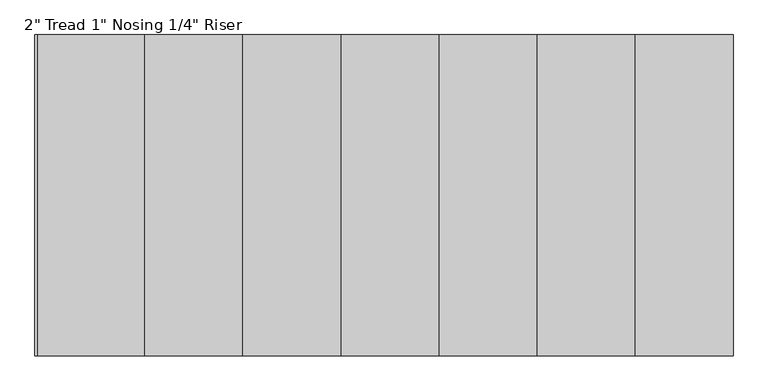
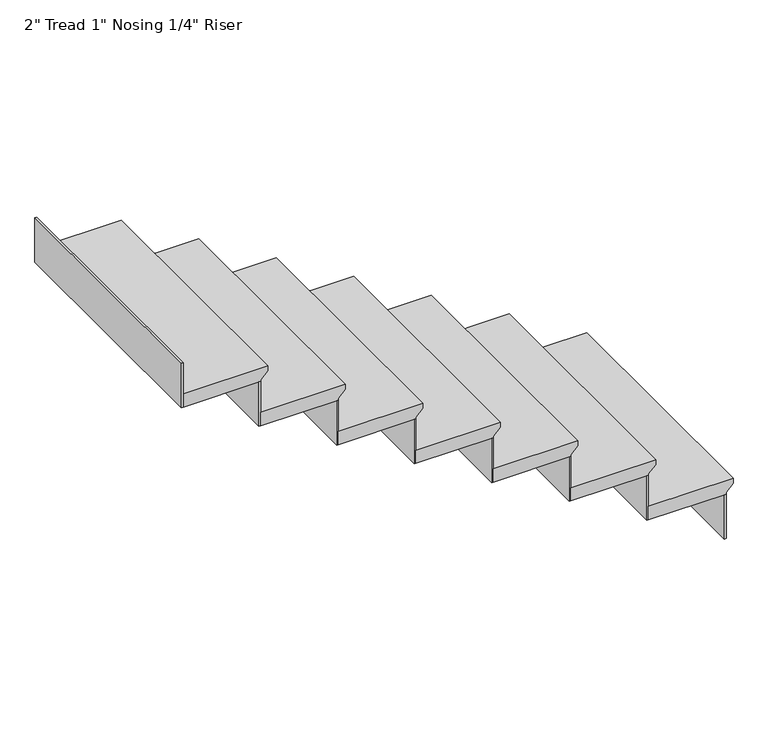
"""IFC4 building model written with IfcOpenShell, lengths in millimetres: stair flight geometry."""

from ifc_helpers import new_model, si_unit, frame, origin, place, context, project, spatial, polyline, outline, extrude, source, transform, mapped, element, save


def stair_flight_f02a3465(model_context):
    return source(origin(), model_context, "Body", "SweptSolid", [
        extrude(outline(polyline([(4876.8, 678.235938), (4876.8, 373.435938), (4826.0, 373.435938), (4826.0, 652.835938), (4832.35, 652.835938), (4857.75, 678.235938), (4876.8, 678.235938)])), frame((0.0, 1120.5857363, 0.0), z_axis=(0.0, 1.0, 0.0), x_axis=(0.0, 0.0, 1.0)), (0.0, 0.0, 1.0), 914.4),
        extrude(outline(polyline([(646.485938, 2034.9857363), (652.835938, 2034.9857363), (652.835938, 1120.5857363), (646.485938, 1120.5857363), (646.485938, 2034.9857363)])), frame((0.0, 0.0, 4656.6666667), z_axis=(0.0, 0.0, 1.0), x_axis=(1.0, 0.0, 0.0)), (0.0, 0.0, 1.0), 169.3333333),
        extrude(outline(polyline([(367.085938, 2034.9857363), (373.435938, 2034.9857363), (373.435938, 1120.5857363), (367.085938, 1120.5857363), (367.085938, 2034.9857363)])), frame((0.0, 0.0, 4826.0), z_axis=(0.0, 0.0, 1.0), x_axis=(1.0, 0.0, 0.0)), (0.0, 0.0, 1.0), 169.3333333),
        extrude(outline(polyline([(5046.1333333, 398.835938), (5046.1333333, 94.035938), (4995.3333333, 94.035938), (4995.3333333, 373.435938), (5001.6833333, 373.435938), (5027.0833333, 398.835938), (5046.1333333, 398.835938)])), frame((0.0, 1120.5857363, 0.0), z_axis=(0.0, 1.0, 0.0), x_axis=(0.0, 0.0, 1.0)), (0.0, 0.0, 1.0), 914.4),
        extrude(outline(polyline([(87.685938, 2034.9857363), (94.035938, 2034.9857363), (94.035938, 1120.5857363), (87.685938, 1120.5857363), (87.685938, 2034.9857363)])), frame((0.0, 0.0, 4995.3333333), z_axis=(0.0, 0.0, 1.0), x_axis=(1.0, 0.0, 0.0)), (0.0, 0.0, 1.0), 169.3333333),
        extrude(outline(polyline([(5215.4666667, 119.435938), (5215.4666667, -185.364062), (5164.6666667, -185.364062), (5164.6666667, 94.035938), (5171.0166667, 94.035938), (5196.4166667, 119.435938), (5215.4666667, 119.435938)])), frame((0.0, 1120.5857363, 0.0), z_axis=(0.0, 1.0, 0.0), x_axis=(0.0, 0.0, 1.0)), (0.0, 0.0, 1.0), 914.4),
        extrude(outline(polyline([(-191.714062, 2034.9857363), (-185.364062, 2034.9857363), (-185.364062, 1120.5857363), (-191.714062, 1120.5857363), (-191.714062, 2034.9857363)])), frame((0.0, 0.0, 5164.6666667), z_axis=(0.0, 0.0, 1.0), x_axis=(1.0, 0.0, 0.0)), (0.0, 0.0, 1.0), 169.3333333),
        extrude(outline(polyline([(5384.8, -159.964062), (5384.8, -464.764062), (5334.0, -464.764062), (5334.0, -185.364062), (5340.35, -185.364062), (5365.75, -159.964062), (5384.8, -159.964062)])), frame((0.0, 1120.5857363, 0.0), z_axis=(0.0, 1.0, 0.0), x_axis=(0.0, 0.0, 1.0)), (0.0, 0.0, 1.0), 914.4),
        extrude(outline(polyline([(-471.114062, 2034.9857363), (-464.764062, 2034.9857363), (-464.764062, 1120.5857363), (-471.114062, 1120.5857363), (-471.114062, 2034.9857363)])), frame((0.0, 0.0, 5334.0), z_axis=(0.0, 0.0, 1.0), x_axis=(1.0, 0.0, 0.0)), (0.0, 0.0, 1.0), 169.3333333),
        extrude(outline(polyline([(5554.1333333, -439.364062), (5554.1333333, -744.164062), (5503.3333333, -744.164062), (5503.3333333, -464.764062), (5509.6833333, -464.764062), (5535.0833333, -439.364062), (5554.1333333, -439.364062)])), frame((0.0, 1120.5857363, 0.0), z_axis=(0.0, 1.0, 0.0), x_axis=(0.0, 0.0, 1.0)), (0.0, 0.0, 1.0), 914.4),
        extrude(outline(polyline([(-750.514062, 2034.9857363), (-744.164062, 2034.9857363), (-744.164062, 1120.5857363), (-750.514062, 1120.5857363), (-750.514062, 2034.9857363)])), frame((0.0, 0.0, 5503.3333333), z_axis=(0.0, 0.0, 1.0), x_axis=(1.0, 0.0, 0.0)), (0.0, 0.0, 1.0), 169.3333333),
        extrude(outline(polyline([(5723.4666667, -718.764062), (5723.4666667, -1023.564062), (5672.6666667, -1023.564062), (5672.6666667, -744.164062), (5679.0166667, -744.164062), (5704.4166667, -718.764062), (5723.4666667, -718.764062)])), frame((0.0, 1120.5857363, 0.0), z_axis=(0.0, 1.0, 0.0), x_axis=(0.0, 0.0, 1.0)), (0.0, 0.0, 1.0), 914.4),
        extrude(outline(polyline([(-1029.914062, 2034.9857363), (-1023.564062, 2034.9857363), (-1023.564062, 1120.5857363), (-1029.914062, 1120.5857363), (-1029.914062, 2034.9857363)])), frame((0.0, 0.0, 5672.6666667), z_axis=(0.0, 0.0, 1.0), x_axis=(1.0, 0.0, 0.0)), (0.0, 0.0, 1.0), 169.3333333),
        extrude(outline(polyline([(-1309.314062, 2034.9857363), (-1302.964062, 2034.9857363), (-1302.964062, 1120.5857363), (-1309.314062, 1120.5857363), (-1309.314062, 2034.9857363)])), frame((0.0, 0.0, 5842.0), z_axis=(0.0, 0.0, 1.0), x_axis=(1.0, 0.0, 0.0)), (0.0, 0.0, 1.0), 169.3333333),
        extrude(outline(polyline([(5892.8, -998.164062), (5892.8, -1302.964062), (5842.0, -1302.964062), (5842.0, -1023.564062), (5848.35, -1023.564062), (5873.75, -998.164062), (5892.8, -998.164062)])), frame((0.0, 1120.5857363, 0.0), z_axis=(0.0, 1.0, 0.0), x_axis=(0.0, 0.0, 1.0)), (0.0, 0.0, 1.0), 914.4),
    ])


if __name__ == "__main__":
    model = new_model("IFC4")
    model_context = context("Model", 3, world=origin())
    ifc_project = project(units=[si_unit("LENGTHUNIT", "METRE", prefix="MILLI")], contexts=[model_context])
    site = spatial("IfcSite", under=ifc_project)
    building = spatial("IfcBuilding", under=site)
    placement = place(None, origin())
    stair_flight_shape = stair_flight_f02a3465(model_context)
    element("IfcStairFlight", 1, ObjectType="2\" Tread 1\" Nosing 1/4\" Riser", at=placement, inside=building, context=model_context, shape_type="MappedRepresentation", body=[
        mapped(stair_flight_shape, transform((0.0, 0.0, 0.0), x_axis=(1.0, 0.0, 0.0), y_axis=(0.0, 1.0, 0.0), z_axis=(0.0, 0.0, 1.0))),
    ])
    save(model, "model.ifc")

# Revit data of these elements
# Element 1 (IfcStairFlight, "2\" Tread 1\" Nosing 1/4\" Riser")
#   Materials on its faces: "BURGUNDY COLOUR"
# Materials
#   "BURGUNDY COLOUR": class "Generic", colour RGB 120 120 120, transparency 0, Cost = 0
